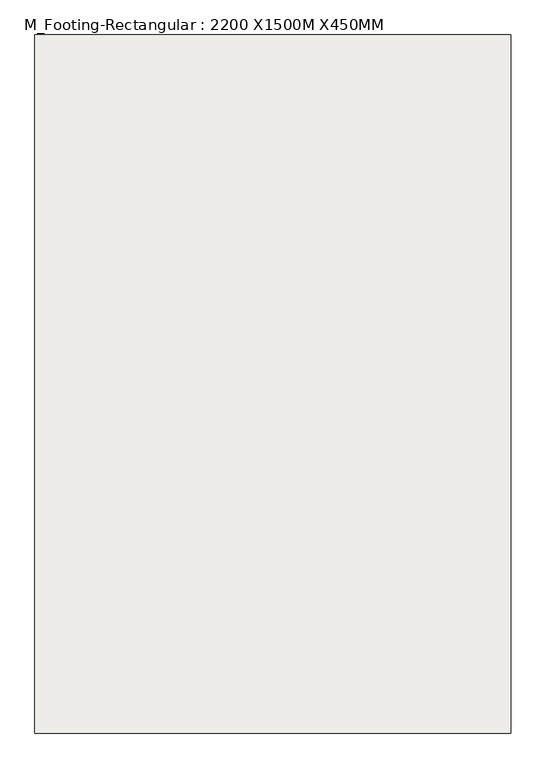
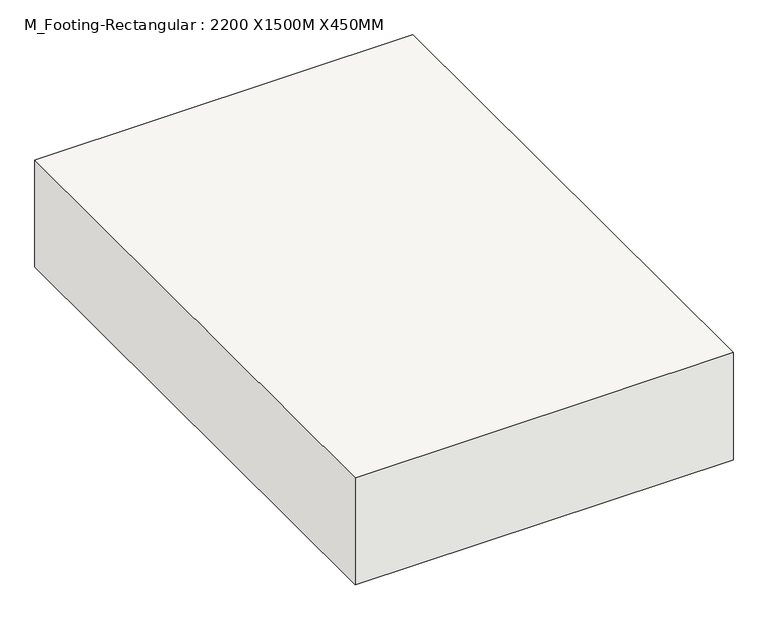
"""IFC4 building model written with IfcOpenShell, lengths in millimetres: slab geometry, M_Footing-Rectangular : 2200 X1500M X450MM."""

from ifc_helpers import new_model, si_unit, frame, origin, place, context, project, spatial, polyline, outline, extrude, source, transform, mapped, element, save


def m_footing_rectangular_2200_x1500m_x450mm_63325679(model_context):
    return source(origin(), model_context, "Body", "SweptSolid", [
        extrude(outline(polyline([(750.0, 1100.0), (750.0, -1100.0), (-750.0, -1100.0), (-750.0, 1100.0), (750.0, 1100.0)])), frame((0.0, 0.0, -450.0), z_axis=(0.0, 0.0, 1.0), x_axis=(1.0, 0.0, 0.0)), (0.0, 0.0, 1.0), 450.0),
    ])


if __name__ == "__main__":
    model = new_model("IFC4")
    model_context = context("Model", 3, world=origin())
    ifc_project = project(units=[si_unit("LENGTHUNIT", "METRE", prefix="MILLI")], contexts=[model_context])
    site = spatial("IfcSite", under=ifc_project)
    building = spatial("IfcBuilding", under=site)
    placement = place(None, origin())
    m_footing_rectangular_2200_x1500m_x450mm_shape = m_footing_rectangular_2200_x1500m_x450mm_63325679(model_context)
    element("IfcSlab", 1, ObjectType="M_Footing-Rectangular : 2200 X1500M X450MM", at=placement, inside=building, context=model_context, shape_type="MappedRepresentation", body=[
        mapped(m_footing_rectangular_2200_x1500m_x450mm_shape, transform((0.0, 0.0, 0.0), x_axis=(1.0, 0.0, 0.0), y_axis=(0.0, 1.0, 0.0), z_axis=(0.0, 0.0, 1.0))),
    ])
    save(model, "model.ifc")

# Revit data of these elements
# Type "M_Footing-Rectangular : 2200 X1500M X450MM"
#   Width = 1500 mm
#   Length = 2200 mm
#   Foundation Thickness = 450 mm
#   Structural Material [instance default] = Concrete, Cast-in-Place gray
#   Assembly Code = ""
# Element 1 (IfcSlab, "M_Footing-Rectangular : 2200 X1500M X450MM")
#   Materials on its faces: "Concrete, Cast-in-Place gray"
# Materials
#   "Concrete, Cast-in-Place gray": class "Concrete", colour RGB 192 192 192, transparency 0, Description = "Cast-in-place concrete", Cost = 0
